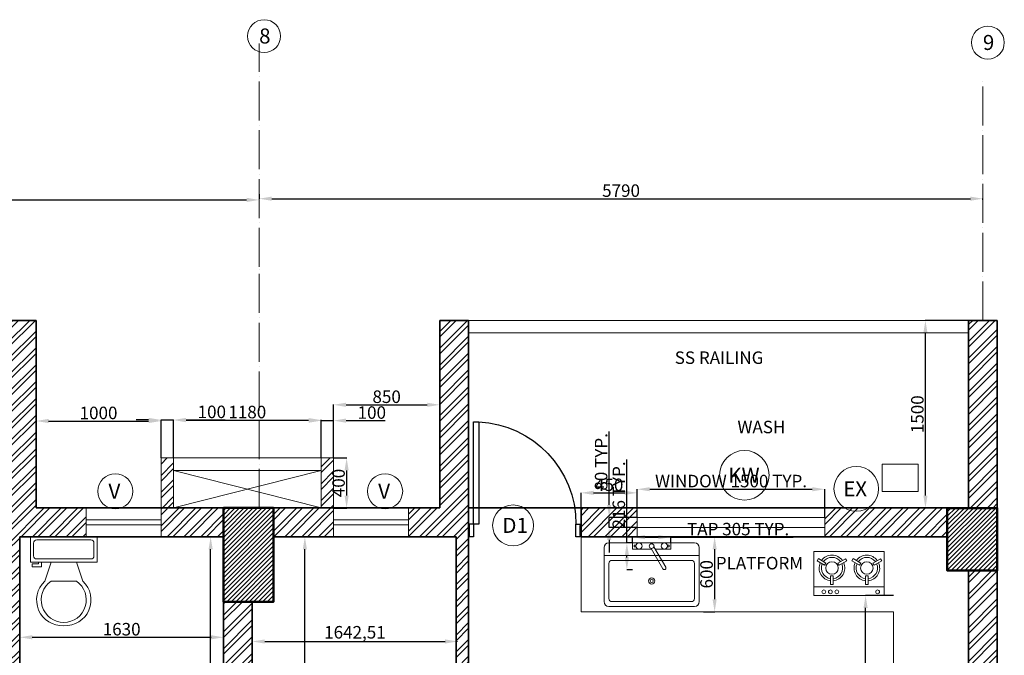
# Model space of a CAD drawing. Units: millimetres. Extents: x -3326 to 29338, y -16792 to 6002.
# Tile 21 of 21: x 21462 to 29338, y 918 to 6002. Entities that reach past the tile are written whole.
import ezdxf

# ---------------------------------------------------------------- set-up
doc = ezdxf.new("R2010")
doc.units = ezdxf.units.MM
doc.header["$PDMODE"] = 35
doc.header["$PDSIZE"] = 5
doc.linetypes.add('ACAD_ISO04W100', pattern=[30, 24, -3, 0, -3])
for name, color, linetype, lineweight in [('A-ANNO-DIMS', 2, 'Continuous', 13), ('A-ANNO-SYMB', 7, 'Continuous', 18), ('A-AREA-IDEN', 7, 'Continuous', 18), ('A-COLS', 1, 'Continuous', 50), ('A-COLS-PATT', 251, 'Continuous', 13), ('A-DOOR', 3, 'Continuous', 25), ('A-EQPM', 9, 'Continuous', 18), ('A-FLOR-CASE', 30, 'Continuous', 18), ('A-FLOR-FIXT', 9, 'Continuous', 18), ('A-FLOR-RAIL', 8, 'Continuous', 20), ('A-FLOR-SHFT', 8, 'Continuous', 18), ('A-GLAZ', 4, 'Continuous', 18), ('A-GRID', 8, 'ACAD_ISO04W100', 13), ('A-GRID-IDEN', 7, 'Continuous', 18), ('A-WALL', 7, 'Continuous', 35), ('A-WALL-PATT', 252, 'Continuous', 13), ('txt', 7, 'Continuous', 18)]:
    doc.layers.add(name, color=color, linetype=linetype, lineweight=lineweight)
doc.styles.get("Standard").update_dxf_attribs({"font": 'arial.ttf'})
doc.dimstyles.new('ISO-25', dxfattribs={"dimtxt": 100, "dimasz": 100, "dimexe": 1.25, "dimexo": 0.625, "dimtad": 1, "dimtxsty": 'Standard', "dimcen": 2.5, "dimadec": 0, "dimazin": 0, "dimtfac": 1, "dimtmove": 0, "dimatfit": 3, "dimfxl": 1, "dimarcsym": 0})
pattern_1 = [(45, (-10476.65, 1e-12), (-67.35192, 67.35192), []), (45, (-10431.74, 1e-12), (-67.35192, 67.35192), [])]

# ---------------------------------------------------------------- blocks, each defined once
blk = doc.blocks.new('A$C0CE462CD')
for p, q in [((860, 100), (860, 0)), ((860, 0), (893.9, 0))]:
    blk.add_line(p, q)
for points in [[(860, 100), (860, 920), (818.4, 920), (818.4, 100)], [(0, 10), (6.1, 10), (6.1, 90), (0, 90)], [(893.9, 10), (900, 10), (900, 90), (893.9, 90)]]:
    blk.add_lwpolyline(points, close=True)
for points in [[(6.1, 0), (40, 0), (40, 100), (6.1, 100)], [(6.1, 100), (6.1, 0)], [(860, 100), (893.9, 100), (893.9, 0)]]:
    blk.add_lwpolyline(points)
blk.add_arc((859.1, 101.9), 819.1, 92.8508, 180.13091)
blk = doc.blocks.new('*U5')
for p, q in [((9.5, -6), (9.5, -2)), ((-10, -8.5), (-8, -8.5)), ((-10, -9.5), (-10, -8.5)), ((-8, -8.5), (-8, -8)), ((-7, -8), (-7, -9.5)), ((-4, -8), (-6, -14)), ((4, -8), (6, -14)), ((-7, -9.5), (-10, -9.5)), ((4, -14), (-4, -14))]:
    blk.add_line(p, q)
blk.add_lwpolyline([(10.5, -8), (10.5, 0), (-10.5, 0), (-10.5, -8)], close=True)
for points in [[(-9.5, -2), (-9.5, -6)], [(8.5, -1), (-8.5, -1)], [(-8.5, -7), (8.5, -7)]]:
    blk.add_lwpolyline(points)
for centre, radius, start, end in [((-8.625, -1.875), 0.8839, 81.8699, 188.1301), ((8.625, -1.875), 0.8839, 351.8699, 98.1301), ((-8.625, -6.125), 0.8839, 171.869898, 278.1301), ((8.625, -6.125), 0.8839, 261.8699, 8.1301), ((-0.4772, -19.9188), 8.0953, 133.01722, 273.38), ((0.0374, -19.8731), 7.127, 124.50543, 269.7), ((-0.0373, -19.8731), 7.127, 270.3, 55.4946), ((0.4773, -19.9188), 8.0953, 266.62, 46.9828)]:
    blk.add_arc(centre, radius, start, end)
blk = doc.blocks.new('Sink-single - 30 in top')
blk.add_line((-15, -3.999996), (15, -3.999996))
for points in [[(-13.5, 0), (13.5, 0)], [(-15, -18.499996), (-15, -1.5)], [(15, -1.5), (15, -18.499996)], [(-12.5, -5.499996), (12.5, -5.499996)], [(-13.5, -17.499996), (-13.5, -6.499996)], [(13.5, -6.499996), (13.5, -17.499996)], [(12.5, -18.499996), (-12.5, -18.499996)], [(13.5, -19.999996), (-13.5, -19.999996)]]:
    blk.add_lwpolyline(points)
for radius in [1, 0.5]:
    blk.add_circle((0, -11.999996), radius)
for centre, radius, start, end in [((-13.5, -1.5), 1.5, 90, 180), ((13.5, -1.5), 1.5, 0, 90), ((-12.5, -6.499996), 1, 90, 180), ((12.5, -6.499996), 1, 0, 90), ((-13.5, -18.499996), 1.5, 180, 270), ((-12.5, -17.499996), 1, 180, 270), ((12.5, -17.499996), 1, 270, 0), ((13.5, -18.499996), 1.5, 270, 0)]:
    blk.add_arc(centre, radius, start, end)
blk = doc.blocks.new('Faucet - kit sink top')
for p, q in [((-5.5, -0.75), (-5.5, -1.25)), ((-4.94278, -0.75), (-5.5, -0.75)), ((-5.5, -1.25), (-4.94278, -1.25)), ((-0.14775, -1.7441), (3.56698, -8.1782)), ((4.43301, -7.6782), (0.71828, -1.2441)), ((4.94278, -0.75), (5.5, -0.75)), ((5.5, -1.25), (4.94278, -1.25)), ((5.5, -0.75), (5.5, -1.25))]:
    blk.add_line(p, q)
blk.add_lwpolyline([(-0.00587, -2), (-6, -2), (-6, 0), (6, 0), (6, -2), (1.15195, -2)])
for centre, radius in [((-4, -1), 1), ((4, -1), 1), ((0, -1), 0.75)]:
    blk.add_circle(centre, radius)
blk.add_arc((4, -7.9282), 0.5, 210, 30)
blk = doc.blocks.new('*D98')
at = {"layer": 'A-ANNO-DIMS', "color": 0, "lineweight": -2, "transparency": 16777216}
for p, q in [((29051.7, 3596), (28706, 3596)), ((28707.2, 2196), (28707.2, 3496)), ((29051.7, 2096), (28706, 2096))]:
    blk.add_line(p, q, dxfattribs=at)
at = {"layer": 'A-ANNO-DIMS', "color": 0, "transparency": 16777216}
for points in [[(28690.6, 3496), (28723.9, 3496), (28707.2, 3596)], [(28690.6, 2196), (28723.9, 2196), (28707.2, 2096)]]:
    blk.add_solid(points, dxfattribs=at)
at = {"layer": 'Defpoints', "color": 0, "transparency": 16777216}
for p in [(28707.2, 3596), (29052.3, 3596), (29052.3, 2096)]:
    blk.add_point(p, dxfattribs=at)
at = {"layer": 'A-ANNO-DIMS', "color": 0, "transparency": 16777216, "insert": (28655.6, 2846), "char_height": 100, "attachment_point": 5, "rotation": 90}
blk.add_mtext('1500', dxfattribs=at)
blk = doc.blocks.new('*D99')
at = {"layer": 'A-ANNO-DIMS', "color": 0, "lineweight": -2, "transparency": 16777216}
for p, q in [((26931, 1866), (27022.1, 1866)), ((27020.9, 1766), (27020.9, 1366)), ((26931, 1266), (27022.1, 1266))]:
    blk.add_line(p, q, dxfattribs=at)
at = {"layer": 'A-ANNO-DIMS', "color": 0, "transparency": 16777216}
for points in [[(27004.2, 1766), (27037.5, 1766), (27020.9, 1866)], [(27004.2, 1366), (27037.5, 1366), (27020.9, 1266)]]:
    blk.add_solid(points, dxfattribs=at)
at = {"layer": 'Defpoints', "color": 0, "transparency": 16777216}
for p in [(26930.3, 1866), (26930.3, 1266), (27020.9, 1266)]:
    blk.add_point(p, dxfattribs=at)
at = {"layer": 'A-ANNO-DIMS', "color": 0, "transparency": 16777216, "insert": (26969.2, 1566), "char_height": 100, "attachment_point": 5, "rotation": 90}
blk.add_mtext('600', dxfattribs=at)
blk = doc.blocks.new('*D103')
at = {"layer": 'A-ANNO-DIMS', "color": 0, "lineweight": -2, "transparency": 16777216}
for p, q in [((28451.7, 1396.4), (28227.4, 1396.4)), ((28228.6, -1834), (28228.6, 1296.4)), ((28451.7, -1934), (28227.4, -1934))]:
    blk.add_line(p, q, dxfattribs=at)
at = {"layer": 'A-ANNO-DIMS', "color": 0, "transparency": 16777216}
for points in [[(28212, 1296.4), (28245.3, 1296.4), (28228.6, 1396.4)], [(28212, -1834), (28245.3, -1834), (28228.6, -1934)]]:
    blk.add_solid(points, dxfattribs=at)
at = {"layer": 'Defpoints', "color": 0, "transparency": 16777216}
for p in [(28228.6, 1396.4), (28452.3, 1396.4), (28452.3, -1934)]:
    blk.add_point(p, dxfattribs=at)
at = {"layer": 'A-ANNO-DIMS', "color": 0, "transparency": 16777216, "insert": (28167.9, -268.8), "char_height": 100, "attachment_point": 5, "rotation": 90}
blk.add_mtext('3330,33', dxfattribs=at)
blk = doc.blocks.new('*D104')
at = {"layer": 'A-ANNO-DIMS', "color": 0, "lineweight": -2, "transparency": 16777216}
for p, q in [((25952.3, 2096.7), (25952.3, 2218.5)), ((26052.3, 2217.2), (26302.3, 2217.2)), ((26402.3, 2096.7), (26402.3, 2218.5))]:
    blk.add_line(p, q, dxfattribs=at)
at = {"layer": 'A-ANNO-DIMS', "color": 0, "transparency": 16777216}
for points in [[(26052.3, 2233.9), (26052.3, 2200.5), (25952.3, 2217.2)], [(26302.3, 2233.9), (26302.3, 2200.5), (26402.3, 2217.2)]]:
    blk.add_solid(points, dxfattribs=at)
at = {"layer": 'Defpoints', "color": 0, "transparency": 16777216}
for p in [(26402.3, 2217.2), (25952.3, 2096), (26402.3, 2096)]:
    blk.add_point(p, dxfattribs=at)
at = {"layer": 'A-ANNO-DIMS', "color": 0, "transparency": 16777216, "insert": (26177.3, 2268.9), "char_height": 100, "attachment_point": 5}
blk.add_mtext('450', dxfattribs=at)
blk = doc.blocks.new('*D105')
at = {"layer": 'A-ANNO-DIMS', "color": 0, "lineweight": -2, "transparency": 16777216}
for p, q in [((22692.3, 2496.7), (22692.3, 2800.2)), ((22792.3, 2799), (23772.3, 2799)), ((23872.3, 2496.7), (23872.3, 2800.2))]:
    blk.add_line(p, q, dxfattribs=at)
at = {"layer": 'A-ANNO-DIMS', "color": 0, "transparency": 16777216}
for points in [[(22792.3, 2815.6), (22792.3, 2782.3), (22692.3, 2799)], [(23772.3, 2815.6), (23772.3, 2782.3), (23872.3, 2799)]]:
    blk.add_solid(points, dxfattribs=at)
at = {"layer": 'Defpoints', "color": 0, "transparency": 16777216}
for p in [(23872.3, 2799), (22692.3, 2496), (23872.3, 2496)]:
    blk.add_point(p, dxfattribs=at)
at = {"layer": 'A-ANNO-DIMS', "color": 0, "transparency": 16777216, "insert": (23282.3, 2850.6), "char_height": 100, "attachment_point": 5}
blk.add_mtext('1180', dxfattribs=at)
blk = doc.blocks.new('*D106')
at = {"layer": 'A-ANNO-DIMS', "color": 0, "lineweight": -2, "transparency": 16777216}
for p, q in [((23772.3, 2794.8), (23672.3, 2794.8)), ((23872.3, 2496.7), (23872.3, 2796)), ((23872.3, 2794.8), (23972.3, 2794.8)), ((23972.3, 2496.7), (23972.3, 2796)), ((24072.3, 2794.8), (24384.7, 2794.8))]:
    blk.add_line(p, q, dxfattribs=at)
at = {"layer": 'A-ANNO-DIMS', "color": 0, "transparency": 16777216}
for points in [[(23772.3, 2811.5), (23772.3, 2778.1), (23872.3, 2794.8)], [(24072.3, 2811.5), (24072.3, 2778.1), (23972.3, 2794.8)]]:
    blk.add_solid(points, dxfattribs=at)
at = {"layer": 'Defpoints', "color": 0, "transparency": 16777216}
for p in [(23972.3, 2794.8), (23872.3, 2496), (23972.3, 2496)]:
    blk.add_point(p, dxfattribs=at)
at = {"layer": 'A-ANNO-DIMS', "color": 0, "transparency": 16777216, "insert": (24278.5, 2846.5), "char_height": 100, "attachment_point": 5}
blk.add_mtext('100', dxfattribs=at)
blk = doc.blocks.new('*D107')
at = {"layer": 'A-ANNO-DIMS', "color": 0, "lineweight": -2, "transparency": 16777216}
for p, q in [((22492.3, 2800.2), (22392.3, 2800.2)), ((22592.3, 2496.7), (22592.3, 2801.5)), ((22592.3, 2800.2), (22692.3, 2800.2)), ((22692.3, 2496.7), (22692.3, 2801.5)), ((22792.3, 2800.2), (23104.7, 2800.2))]:
    blk.add_line(p, q, dxfattribs=at)
at = {"layer": 'A-ANNO-DIMS', "color": 0, "transparency": 16777216}
for points in [[(22492.3, 2816.9), (22492.3, 2783.5), (22592.3, 2800.2)], [(22792.3, 2816.9), (22792.3, 2783.5), (22692.3, 2800.2)]]:
    blk.add_solid(points, dxfattribs=at)
at = {"layer": 'Defpoints', "color": 0, "transparency": 16777216}
for p in [(22692.3, 2800.2), (22592.3, 2496), (22692.3, 2496)]:
    blk.add_point(p, dxfattribs=at)
at = {"layer": 'A-ANNO-DIMS', "color": 0, "transparency": 16777216, "insert": (22998.5, 2851.9), "char_height": 100, "attachment_point": 5}
blk.add_mtext('100', dxfattribs=at)
blk = doc.blocks.new('*D108')
at = {"layer": 'A-ANNO-DIMS', "color": 0, "lineweight": -2, "transparency": 16777216}
for p, q in [((21592.3, 2702.3), (21592.3, 2793.1)), ((21692.3, 2791.9), (22492.3, 2791.9)), ((22592.3, 2702.3), (22592.3, 2793.1))]:
    blk.add_line(p, q, dxfattribs=at)
at = {"layer": 'A-ANNO-DIMS', "color": 0, "transparency": 16777216}
for points in [[(21692.3, 2808.5), (21692.3, 2775.2), (21592.3, 2791.9)], [(22492.3, 2808.5), (22492.3, 2775.2), (22592.3, 2791.9)]]:
    blk.add_solid(points, dxfattribs=at)
at = {"layer": 'Defpoints', "color": 0, "transparency": 16777216}
for p in [(22592.3, 2791.9), (21592.3, 2701.7), (22592.3, 2701.7)]:
    blk.add_point(p, dxfattribs=at)
at = {"layer": 'A-ANNO-DIMS', "color": 0, "transparency": 16777216, "insert": (22092.3, 2843.6), "char_height": 100, "attachment_point": 5}
blk.add_mtext('1000', dxfattribs=at)
blk = doc.blocks.new('*D109')
at = {"layer": 'A-ANNO-DIMS', "color": 0, "lineweight": -2, "transparency": 16777216}
for p, q in [((23972.3, 2647), (23972.3, 2922.7)), ((24072.3, 2921.4), (24722.3, 2921.4)), ((24822.3, 2647), (24822.3, 2922.7))]:
    blk.add_line(p, q, dxfattribs=at)
at = {"layer": 'A-ANNO-DIMS', "color": 0, "transparency": 16777216}
for points in [[(24072.3, 2938.1), (24072.3, 2904.8), (23972.3, 2921.4)], [(24722.3, 2938.1), (24722.3, 2904.8), (24822.3, 2921.4)]]:
    blk.add_solid(points, dxfattribs=at)
at = {"layer": 'Defpoints', "color": 0, "transparency": 16777216}
for p in [(24822.3, 2921.4), (23972.3, 2646.4), (24822.3, 2646.4)]:
    blk.add_point(p, dxfattribs=at)
at = {"layer": 'A-ANNO-DIMS', "color": 0, "transparency": 16777216, "insert": (24397.3, 2973.1), "char_height": 100, "attachment_point": 5}
blk.add_mtext('850', dxfattribs=at)
blk = doc.blocks.new('*D110')
at = {"layer": 'A-ANNO-DIMS', "color": 0, "lineweight": -2, "transparency": 16777216}
for p, q in [((23972.9, 2496), (24078.3, 2496)), ((24077, 2396), (24077, 2196)), ((23972.9, 2096), (24078.3, 2096))]:
    blk.add_line(p, q, dxfattribs=at)
at = {"layer": 'A-ANNO-DIMS', "color": 0, "transparency": 16777216}
for points in [[(24060.4, 2396), (24093.7, 2396), (24077, 2496)], [(24060.4, 2196), (24093.7, 2196), (24077, 2096)]]:
    blk.add_solid(points, dxfattribs=at)
at = {"layer": 'Defpoints', "color": 0, "transparency": 16777216}
for p in [(23972.3, 2496), (23972.3, 2096), (24077, 2096)]:
    blk.add_point(p, dxfattribs=at)
at = {"layer": 'A-ANNO-DIMS', "color": 0, "transparency": 16777216, "insert": (24025.4, 2296), "char_height": 100, "attachment_point": 5, "rotation": 90}
blk.add_mtext('400', dxfattribs=at)
blk = doc.blocks.new('*D111')
at = {"layer": 'A-ANNO-DIMS', "color": 0, "lineweight": -2, "transparency": 16777216}
for p, q in [((23322.3, 1029), (23322.3, 1029.6)), ((23422.3, 1028.4), (24864.8, 1028.4)), ((24964.8, 1029), (24964.8, 1029.6))]:
    blk.add_line(p, q, dxfattribs=at)
at = {"layer": 'A-ANNO-DIMS', "color": 0, "transparency": 16777216}
for points in [[(23422.3, 1045), (23422.3, 1011.7), (23322.3, 1028.4)], [(24864.8, 1045), (24864.8, 1011.7), (24964.8, 1028.4)]]:
    blk.add_solid(points, dxfattribs=at)
at = {"layer": 'Defpoints', "color": 0, "transparency": 16777216}
for p in [(23322.3, 1028.4), (24964.8, 1028.4), (24964.8, 1028.4)]:
    blk.add_point(p, dxfattribs=at)
at = {"layer": 'A-ANNO-DIMS', "color": 0, "transparency": 16777216, "insert": (24143.6, 1089.1), "char_height": 100, "attachment_point": 5}
blk.add_mtext('1642,51', dxfattribs=at)
blk = doc.blocks.new('*D112')
at = {"layer": 'A-ANNO-DIMS', "color": 0, "lineweight": -2, "transparency": 16777216}
for p, q in [((23743.4, 1866), (23744, 1866)), ((23742.8, -1634), (23742.8, 1766)), ((23743.4, -1734), (23744, -1734))]:
    blk.add_line(p, q, dxfattribs=at)
at = {"layer": 'A-ANNO-DIMS', "color": 0, "transparency": 16777216}
for points in [[(23726.1, 1766), (23759.4, 1766), (23742.8, 1866)], [(23726.1, -1634), (23759.4, -1634), (23742.8, -1734)]]:
    blk.add_solid(points, dxfattribs=at)
at = {"layer": 'Defpoints', "color": 0, "transparency": 16777216}
for p in [(23742.8, 1866), (23742.8, 1866), (23742.8, -1734)]:
    blk.add_point(p, dxfattribs=at)
at = {"layer": 'A-ANNO-DIMS', "color": 0, "transparency": 16777216, "insert": (23691.1, 66), "char_height": 100, "attachment_point": 5, "rotation": 90}
blk.add_mtext('3600', dxfattribs=at)
blk = doc.blocks.new('*D113')
at = {"layer": 'A-ANNO-DIMS', "color": 0, "lineweight": -2, "transparency": 16777216}
for p, q in [((21462.3, 1061.3), (21462.3, 1060.7)), ((21562.3, 1061.9), (22992.3, 1061.9)), ((23092.3, 1062.5), (23092.3, 1063.2))]:
    blk.add_line(p, q, dxfattribs=at)
at = {"layer": 'A-ANNO-DIMS', "color": 0, "transparency": 16777216}
for points in [[(21562.3, 1078.6), (21562.3, 1045.3), (21462.3, 1061.9)], [(22992.3, 1078.6), (22992.3, 1045.3), (23092.3, 1061.9)]]:
    blk.add_solid(points, dxfattribs=at)
at = {"layer": 'Defpoints', "color": 0, "transparency": 16777216}
for p in [(21462.3, 1061.9), (23092.3, 1061.9), (23092.3, 1061.9)]:
    blk.add_point(p, dxfattribs=at)
at = {"layer": 'A-ANNO-DIMS', "color": 0, "transparency": 16777216, "insert": (22277.3, 1113.6), "char_height": 100, "attachment_point": 5}
blk.add_mtext('1630', dxfattribs=at)
blk = doc.blocks.new('*D114')
at = {"layer": 'A-ANNO-DIMS', "color": 0, "lineweight": -2, "transparency": 16777216}
for p, q in [((23091.7, 1866), (22987.8, 1866)), ((22989, -834), (22989, 1766)), ((23091.7, -934), (22987.8, -934))]:
    blk.add_line(p, q, dxfattribs=at)
at = {"layer": 'A-ANNO-DIMS', "color": 0, "transparency": 16777216}
for points in [[(22972.4, 1766), (23005.7, 1766), (22989, 1866)], [(22972.4, -834), (23005.7, -834), (22989, -934)]]:
    blk.add_solid(points, dxfattribs=at)
at = {"layer": 'Defpoints', "color": 0, "transparency": 16777216}
for p in [(22989, 1866), (23092.3, 1866), (23092.3, -934)]:
    blk.add_point(p, dxfattribs=at)
at = {"layer": 'A-ANNO-DIMS', "color": 0, "transparency": 16777216, "insert": (22937.4, 466), "char_height": 100, "attachment_point": 5, "rotation": 90}
blk.add_mtext('2800', dxfattribs=at)
blk = doc.blocks.new('*D155')
at = {"layer": 'A-ANNO-DIMS', "color": 0, "lineweight": -2, "transparency": 16777216}
for p, q in [((17397.3, 4561.1), (17397.3, 4561.8)), ((17497.3, 4560.5), (23277.3, 4560.5)), ((23377.3, 4561.1), (23377.3, 4561.8))]:
    blk.add_line(p, q, dxfattribs=at)
at = {"layer": 'A-ANNO-DIMS', "color": 0, "transparency": 16777216}
for points in [[(17497.3, 4577.2), (17497.3, 4543.8), (17397.3, 4560.5)], [(23277.3, 4577.2), (23277.3, 4543.8), (23377.3, 4560.5)]]:
    blk.add_solid(points, dxfattribs=at)
at = {"layer": 'Defpoints', "color": 0, "transparency": 16777216}
for p in [(17397.3, 4560.5), (23377.3, 4560.5), (23377.3, 4560.5)]:
    blk.add_point(p, dxfattribs=at)
at = {"layer": 'A-ANNO-DIMS', "color": 0, "transparency": 16777216, "insert": (20387.3, 4612.2), "char_height": 100, "attachment_point": 5}
blk.add_mtext('5980', dxfattribs=at)
blk = doc.blocks.new('*D156')
at = {"layer": 'A-ANNO-DIMS', "color": 0, "lineweight": -2, "transparency": 16777216}
for p, q in [((23377.3, 4606), (23377.3, 4568.8)), ((23477.3, 4570), (29067.3, 4570)), ((29167.3, 4561.1), (29167.3, 4571.3))]:
    blk.add_line(p, q, dxfattribs=at)
at = {"layer": 'A-ANNO-DIMS', "color": 0, "transparency": 16777216}
for points in [[(23477.3, 4586.7), (23477.3, 4553.4), (23377.3, 4570)], [(29067.3, 4586.7), (29067.3, 4553.4), (29167.3, 4570)]]:
    blk.add_solid(points, dxfattribs=at)
at = {"layer": 'Defpoints', "color": 0, "transparency": 16777216}
for p in [(23377.3, 4606.6), (29167.3, 4570), (29167.3, 4560.5)]:
    blk.add_point(p, dxfattribs=at)
at = {"layer": 'A-ANNO-DIMS', "color": 0, "transparency": 16777216, "insert": (26272.3, 4621.7), "char_height": 100, "attachment_point": 5}
blk.add_mtext('5790', dxfattribs=at)
blk = doc.blocks.new('COOKTOP-TWO-BURNER')
for p, q in [((561.3, 350.8), (0, 350.8)), ((0, 0), (0, 350.8)), ((561.3, 0), (561.3, 350.8)), ((26.1, 276.2), (36.6, 294.4)), ((86.6, 241.2), (26.1, 276.2)), ((97.2, 259.4), (36.6, 294.4)), ((86.6, 241.2), (97.2, 259.4)), ((193, 259.4), (253.6, 294.3)), ((193, 259.4), (203.5, 241.1)), ((203.5, 241.1), (264.1, 276.1)), ((253.6, 294.3), (264.1, 276.1)), ((305, 276.2), (315.6, 294.4)), ((365.6, 241.2), (305, 276.2)), ((376.1, 259.4), (315.6, 294.4)), ((365.6, 241.2), (376.1, 259.4)), ((472, 259.4), (532.5, 294.3)), ((472, 259.4), (482.5, 241.1)), ((482.5, 241.1), (543, 276.1)), ((532.5, 294.3), (543, 276.1)), ((134.5, 158.1), (134.5, 88.2)), ((155.6, 158.1), (134.5, 158.1)), ((155.6, 158.1), (155.5, 88.2)), ((413.5, 158.1), (413.4, 88.2)), ((434.5, 158.1), (413.5, 158.1)), ((434.5, 158.1), (434.5, 88.2)), ((155.5, 88.2), (134.5, 88.2)), ((434.5, 88.2), (413.4, 88.2)), ((561.3, 70.2), (0, 70.2)), ((561.3, 0), (0, 0))]:
    blk.add_line(p, q)
at = {"extrusion": (0, 0, -1)}
for centre, major_axis, start_param, end_param in [((145.1, 219.6), (-0.2, 102.8), -0.942584, 0.946692), ((424, 219.6), (0, 102.8), -0.944011, 0.945266), ((145.1, 219.6), (-0.1, 102.8), 3.2451, 5.134376), ((145.1, 219.6), (-60.3, 60.3), 4.051123, 5.898002), ((145.1, 219.6), (-60.3, 60.3), 6.145519, 7.992397), ((145.1, 219.6), (-35.5, 35.5), 2.356194490192311, 8.639379797371898), ((145.1, 219.6), (0.1, 102.8), 1.148752, 3.038029), ((145.1, 219.6), (60.3, 60.3), 0.385932, 2.23281), ((424, 219.6), (0, 102.8), 3.244173, 5.13345), ((424, 219.6), (60.3, 60.3), 2.480327, 4.327205), ((424, 219.6), (-60.3, 60.3), 6.145519, 7.992397), ((424, 219.6), (-35.5, 35.5), 2.356194490192306, 8.639379797371893), ((424, 219.6), (0.1, 102.8), 1.14879, 3.038067), ((424, 219.6), (60.3, 60.3), 0.385932, 2.23281), ((79.9, 28.7), (-10.8, 10.8), 2.356194490192189, 8.639379797371776), ((132.6, 28.7), (-10.8, 10.8), 2.356194490192189, 8.639379797371776), ((184.2, 28.7), (-10.8, 10.8), 2.356194490192189, 8.639379797371776), ((510, 28.7), (-10.8, 10.8), 2.356194490192189, 8.639379797371776)]:
    blk.add_ellipse(centre, major_axis=major_axis, ratio=1, start_param=start_param, end_param=end_param, dxfattribs=at)
blk = doc.blocks.new('TAG-D1')
blk.add_circle((163.3, 163.3), 163.3)
at = {"insert": (78, 223.5), "char_height": 120, "attachment_point": 1}
blk.add_mtext_dynamic_manual_height_columns('D1', width=137.943, gutter_width=12.5, heights=[0], dxfattribs=at)
blk = doc.blocks.new('TAG-KW')
blk.add_circle((198.2, 198.2), 198.2)
at = {"insert": (70.3, 258.2), "char_height": 120, "attachment_point": 1}
blk.add_mtext_dynamic_manual_height_columns('KW', width=376.575, gutter_width=12.5, heights=[0], dxfattribs=at)
blk = doc.blocks.new('TAG-V')
blk.add_circle((140.7, 140.7), 140.7)
at = {"insert": (85.8, 200.7), "char_height": 120, "attachment_point": 1}
blk.add_mtext_dynamic_manual_height_columns('V', width=129.836, gutter_width=12.5, heights=[0], dxfattribs=at)
blk = doc.blocks.new('GLAZ-600x40')
for p, q in [((600, 40), (0, 40)), ((600, 0), (0, 0))]:
    blk.add_line(p, q)
blk = doc.blocks.new('GLAZ-1500x80')
for p, q in [((0, 80), (1500, 80)), ((0, 0), (1500, 0))]:
    blk.add_line(p, q)
blk = doc.blocks.new('*D207')
at = {"layer": 'A-ANNO-DIMS', "color": 0, "lineweight": -2, "transparency": 16777216}
for p, q in [((26402.3, 2021.7), (26402.3, 2247.3)), ((26502.3, 2246), (27802.3, 2246)), ((27902.3, 2021.7), (27902.3, 2247.3))]:
    blk.add_line(p, q, dxfattribs=at)
at = {"layer": 'A-ANNO-DIMS', "color": 0, "transparency": 16777216}
for points in [[(26502.3, 2262.7), (26502.3, 2229.4), (26402.3, 2246)], [(27802.3, 2262.7), (27802.3, 2229.4), (27902.3, 2246)]]:
    blk.add_solid(points, dxfattribs=at)
at = {"layer": 'Defpoints', "color": 0, "transparency": 16777216}
for p in [(27902.3, 2246), (26402.3, 2021), (27902.3, 2021)]:
    blk.add_point(p, dxfattribs=at)
at = {"layer": 'A-ANNO-DIMS', "color": 0, "transparency": 16777216, "insert": (27152.3, 2298.4), "char_height": 100, "attachment_point": 5}
blk.add_mtext('WINDOW 1500 TYP.', dxfattribs=at)
blk = doc.blocks.new('*D208')
at = {"layer": 'A-ANNO-DIMS', "color": 0, "lineweight": -2, "transparency": 16777216}
for p, q in [((26177.3, 2121), (26177.3, 2709.2)), ((26401.7, 2021), (26176.1, 2021)), ((26177.3, 1941), (26177.3, 2021)), ((26401.7, 1941), (26176.1, 1941)), ((26177.3, 1841), (26177.3, 1741))]:
    blk.add_line(p, q, dxfattribs=at)
at = {"layer": 'A-ANNO-DIMS', "color": 0, "transparency": 16777216}
for points in [[(26160.6, 2121), (26194, 2121), (26177.3, 2021)], [(26160.6, 1841), (26194, 1841), (26177.3, 1941)]]:
    blk.add_solid(points, dxfattribs=at)
at = {"layer": 'Defpoints', "color": 0, "transparency": 16777216}
for p in [(26177.3, 2021), (26402.3, 2021), (26402.3, 1941)]:
    blk.add_point(p, dxfattribs=at)
at = {"layer": 'A-ANNO-DIMS', "color": 0, "transparency": 16777216, "insert": (26125.6, 2465.1), "char_height": 100, "attachment_point": 5, "rotation": 90}
blk.add_mtext('80 TYP.', dxfattribs=at)
blk = doc.blocks.new('*D223')
at = {"layer": 'A-ANNO-DIMS', "color": 0, "lineweight": -2, "transparency": 16777216}
for p, q in [((26364.7, 1817.6), (26364.7, 1863.9)), ((26464.7, 1862.7), (26569.5, 1862.7)), ((26669.5, 1817.6), (26669.5, 1863.9)), ((26669.5, 1862.7), (27648.2, 1862.7))]:
    blk.add_line(p, q, dxfattribs=at)
at = {"layer": 'A-ANNO-DIMS', "color": 0, "transparency": 16777216}
for points in [[(26464.7, 1879.4), (26464.7, 1846), (26364.7, 1862.7)], [(26569.5, 1879.4), (26569.5, 1846), (26669.5, 1862.7)]]:
    blk.add_solid(points, dxfattribs=at)
at = {"layer": 'Defpoints', "color": 0, "transparency": 16777216}
for p in [(26364.7, 1817), (26669.5, 1862.7), (26669.5, 1817)]:
    blk.add_point(p, dxfattribs=at)
at = {"layer": 'A-ANNO-DIMS', "color": 0, "transparency": 16777216, "insert": (27208.8, 1914.4), "char_height": 100, "attachment_point": 5}
blk.add_mtext('TAP 305 TYP.', dxfattribs=at)
blk = doc.blocks.new('*D224')
at = {"layer": 'A-ANNO-DIMS', "color": 0, "lineweight": -2, "transparency": 16777216}
for p, q in [((26318.9, 1817), (26318.9, 2484.4)), ((26364, 1817), (26317.7, 1817)), ((26318.9, 1701.1), (26318.9, 1717)), ((26364, 1601.1), (26317.7, 1601.1))]:
    blk.add_line(p, q, dxfattribs=at)
at = {"layer": 'A-ANNO-DIMS', "color": 0, "transparency": 16777216}
for points in [[(26302.3, 1717), (26335.6, 1717), (26318.9, 1817)], [(26302.3, 1701.1), (26335.6, 1701.1), (26318.9, 1601.1)]]:
    blk.add_solid(points, dxfattribs=at)
at = {"layer": 'Defpoints', "color": 0, "transparency": 16777216}
for p in [(26318.9, 1817), (26364.7, 1817), (26364.7, 1601.1)]:
    blk.add_point(p, dxfattribs=at)
at = {"layer": 'A-ANNO-DIMS', "color": 0, "transparency": 16777216, "insert": (26267.3, 2200.7), "char_height": 100, "attachment_point": 5, "rotation": 90}
blk.add_mtext('216 TYP.', dxfattribs=at)

msp = doc.modelspace()

# ---------------------------------------------------------------- hatches: boundary and pattern name
at = {"layer": 'A-COLS-PATT'}
h = msp.add_hatch(dxfattribs=at)
h.set_pattern_fill('ANSI31', color=256, scale=8)
h.set_pattern_definition([(45, (-18946.33, 12265.585), (-17.960512, 17.960512), [])])
h.paths.add_polyline_path([(23492.301, 2096.048), (23092.301, 2096.048), (23092.301, 1346.048), (23492.301, 1346.048)])
h = msp.add_hatch(dxfattribs=at)
h.set_pattern_fill('ANSI31', color=256, scale=8)
h.set_pattern_definition([(45, (-15733.41, 7308.703), (-17.960512, 17.960512), [])])
h.paths.add_polyline_path([(28882.301, 2095.065), (28882.301, 1595.065), (29282.301, 1595.065), (29282.301, 2095.065)])
at = {"layer": 'A-WALL-PATT'}
h = msp.add_hatch(dxfattribs=at)
h.set_pattern_fill('ANSI32', color=256, scale=10)
h.set_pattern_definition(pattern_1)
h.paths.add_polyline_path([(29282.301, -7283.952), (28882.301, -7283.952), (28882.301, -7383.952), (29052.301, -7383.952), (29052.301, -10763.952), (29282.301, -10763.952)])
h.paths.add_polyline_path([(29282.301, -11263.952), (29052.301, -11263.952), (29052.301, -12763.952), (29282.301, -12763.952)])
h.paths.add_polyline_path([(25052.301, -11263.952), (25652.301, -11263.952), (25652.301, -11123.904), (25652.289, -11123.904), (25652.289, -11033.952), (25052.301, -11033.952), (24572.301, -11033.952), (24572.301, -11263.952), (24822.301, -11263.952), (24822.301, -12763.952), (25052.301, -12763.952)])
h.paths.add_polyline_path([(26902.301, -11033.952), (26552.301, -11033.952), (26552.301, -11263.952), (26902.301, -11263.952)])
h.paths.add_polyline_path([(21992.301, -6683.952), (21362.301, -6683.952), (17512.301, -6683.952), (17512.301, -6783.952), (21362.301, -6783.952), (21992.301, -6783.952)])
h.paths.add_polyline_path([(17512.301, -7283.952), (17282.301, -7283.952), (17282.301, -12163.952), (17512.301, -12163.952), (17512.301, -11263.952), (18112.301, -11263.952), (18112.301, -11033.952), (17512.301, -11033.952)])
h.paths.add_polyline_path([(21462.301, -8211.864), (21462.064, -8211.864), (21462.064, -8142.609), (21462.301, -8133.952), (21362.301, -8133.952), (21362.301, -8233.952), (21362.301, -11033.952), (21162.301, -11033.952), (21162.301, -11263.952), (21362.301, -11263.952), (21362.301, -12763.952), (21592.301, -12763.952), (21592.301, -11263.952), (21992.301, -11263.952), (21992.301, -11033.952), (21592.301, -11033.952), (21462.301, -11033.952)])
h.paths.add_polyline_path([(24152.301, -8133.952), (23322.301, -8133.952), (23322.301, -7433.952), (23092.301, -7433.952), (23092.301, -8133.952), (22241.021, -8133.952), (22241.021, -8142.609), (22241.182, -8142.609), (22241.182, -8211.864), (22241.021, -8233.952), (23092.301, -8233.952), (23092.301, -10513.206), (23322.301, -10513.206), (23322.301, -8233.952), (24152.301, -8233.952)])
h.paths.add_polyline_path([(25052.301, -8233.952), (25052.301, -8133.952), (24952.301, -8133.952), (24952.301, -11033.952), (25052.301, -11033.952)])
h.paths.add_polyline_path([(23972.301, -11033.952), (23493.251, -11033.952), (23493.251, -11263.952), (23972.301, -11263.952)])
h.paths.add_polyline_path([(23092.301, -11033.952), (22592.301, -11033.952), (22592.301, -11263.952), (23092.301, -11263.952)])
h.paths.add_polyline_path([(28882.301, -11033.952), (28702.301, -11033.952), (28702.301, -11263.952), (28882.301, -11263.952)])
h.paths.add_polyline_path([(17512.301, -3883.952), (17387.589, -3883.952), (17387.589, -3888.07), (17282.301, -3888.07), (17282.301, -6683.952), (17512.301, -6683.952)])
h.paths.add_polyline_path([(21462.301, -2183.952), (21362.301, -2183.952), (21362.301, -2383.952), (17282.301, -2383.952), (17282.301, -2483.952), (17512.301, -2483.952), (21462.301, -2483.952)])
h.paths.add_polyline_path([(17512.301, -2483.952), (17282.301, -2483.952), (17282.301, -2833.952), (17512.301, -2833.952)])
h.paths.add_polyline_path([(21462.301, 1866.048), (21992.301, 1866.048), (21992.301, 2096.048), (21592.301, 2096.048), (21592.301, 3596.048), (21362.301, 3596.048), (21362.301, 1866.048), (21362.301, -1283.952), (21462.301, -1283.952)])
h.paths.add_polyline_path([(17512.301, 1496.048), (17282.301, 1496.048), (17282.301, -1983.952), (17612.301, -1983.952), (17612.301, -1883.952), (17512.301, -1883.952)])
h.paths.add_polyline_path([(17512.301, 3596.048), (17282.301, 3596.048), (17282.301, 2096.048), (17512.301, 2096.048)])
h.paths.add_polyline_path([(18135.023, 2096.048), (17685.023, 2096.048), (17685.023, 1866.048), (18135.023, 1866.048), (18135.023, 1876.048), (18128.942, 1876.048), (18128.942, 1956.048), (18135.023, 1956.048)])
h.paths.add_polyline_path([(19385.023, 2096.048), (19035.023, 2096.048), (19035.023, 1866.048), (19385.023, 1866.048)])
h.paths.add_polyline_path([(21362.301, 2096.048), (21185.023, 2096.048), (21185.023, 1866.048), (21362.301, 1866.048)])
h.paths.add_polyline_path([(23092.301, 2096.048), (22592.301, 2096.048), (22592.301, 1866.048), (23092.301, 1866.048)])
h.paths.add_polyline_path([(23972.301, 2096.048), (23492.301, 2096.048), (23492.301, 1866.048), (23972.301, 1866.048)])
h.paths.add_polyline_path([(23972.301, 2496.048), (23872.301, 2496.048), (23872.301, 2096.048), (23972.301, 2096.048)])
h.paths.add_polyline_path([(22692.301, 2496.048), (22592.301, 2496.048), (22592.301, 2096.048), (22692.301, 2096.048)])
h.paths.add_polyline_path([(23322.301, 1346.048), (23092.301, 1346.048), (23092.301, -1733.952), (23322.301, -1733.952)])
h.paths.add_polyline_path([(23092.301, -933.952), (22262.301, -933.952), (22262.301, -1033.952), (23092.301, -1033.952)])
h.paths.add_polyline_path([(24952.301, -1433.952), (24952.301, -1733.952), (23492.301, -1733.952), (23492.301, -1833.952), (24952.301, -1833.952), (24952.301, -2483.952), (25052.301, -2483.952), (25052.301, -2466.23), (25049.26, -2466.23), (25049.26, -2386.23), (25049.941, -1433.952)])
h.paths.add_polyline_path([(22692.301, -11263.952), (22592.301, -11263.952), (22592.301, -11663.952), (22692.301, -11663.952)])
h.paths.add_polyline_path([(23972.301, -11263.952), (23872.301, -11263.952), (23872.301, -11663.952), (23972.301, -11663.952)])
h = msp.add_hatch(dxfattribs=at)
h.set_pattern_fill('ANSI32', color=256, scale=10)
h.set_pattern_definition(pattern_1)
h.paths.add_polyline_path([(29282.301, 3596.048), (29052.301, 3596.048), (29052.301, 2095.065), (29282.301, 2095.065)])
h.paths.add_polyline_path([(25052.301, 3596.048), (24822.301, 3596.048), (24822.301, 2096.048), (24572.301, 2096.048), (24572.301, 1866.048), (24952.301, 1866.048), (24952.301, -633.952), (24972.008, -633.952), (24972.008, -631.026), (25043.379, -631.026), (25052.301, -633.952), (25052.301, 1866.048), (25052.301, 1876.048), (25051.713, 1876.048), (25051.713, 1956.048)])
h.paths.add_polyline_path([(29282.301, 1595.065), (29052.301, 1595.065), (29052.301, -1883.676), (29282.301, -1883.676), (29282.301, 336.048)])
h.paths.add_polyline_path([(28882.301, 2096.048), (27902.301, 2096.048), (27902.301, 1866.048), (28882.301, 1866.048)])
h.paths.add_polyline_path([(26402.301, 2096.048), (25952.301, 2096.048), (25952.301, 1866.048), (26402.301, 1866.048)])
h.paths.add_polyline_path([(28882.301, -2383.952), (25952.301, -2383.952), (25952.301, -2483.952), (27152.301, -2483.952), (27152.301, -2683.952), (27382.301, -2683.952), (27382.301, -2483.952), (28882.301, -2483.952)])

# ---------------------------------------------------------------- linework, layer by layer
at = {"layer": 'A-ANNO-SYMB'}
msp.add_circle((28154.444, 2249.364), 178.636, dxfattribs=at)
at = {"layer": 'A-COLS'}
for points in [[(23092.301, 2096.048), (23492.301, 2096.048), (23492.301, 1346.048), (23092.301, 1346.048)], [(28882.301, 2095.065), (29282.301, 2095.065), (29282.301, 1595.065), (28882.301, 1595.065)]]:
    msp.add_lwpolyline(points, close=True, dxfattribs=at)
at = {"layer": 'A-EQPM'}
msp.add_lwpolyline([(28361.2, 2446.539), (28649.928, 2446.539), (28649.928, 2227.788), (28361.2, 2227.788)], close=True, dxfattribs=at)
at = {"layer": 'A-FLOR-CASE'}
for p, q in [((25952.301, 1866.048), (25952.301, 1266.048)), ((25952.301, 1266.048), (28452.301, 1266.048)), ((28452.301, -1933.952), (28452.301, 1266.048))]:
    msp.add_line(p, q, dxfattribs=at)
at = {"layer": 'A-FLOR-RAIL'}
for p, q in [((29052.301, 3596.048), (25052.301, 3596.048)), ((29052.301, 3496.048), (25052.301, 3496.048))]:
    msp.add_line(p, q, dxfattribs=at)
at = {"layer": 'A-FLOR-SHFT'}
for p, q in [((22592.301, 2096.048), (22592.301, 2496.048)), ((22592.301, 2496.048), (22692.301, 2496.048)), ((22692.301, 2496.048), (22692.301, 2096.048)), ((22692.301, 2496.048), (23872.301, 2496.048)), ((23972.301, 2496.048), (23872.301, 2496.048)), ((23872.301, 2496.048), (23872.301, 2096.048)), ((23972.301, 2096.048), (23972.301, 2496.048)), ((22692.301, 2396.048), (23872.301, 2396.048)), ((22692.301, 2096.048), (23872.301, 2396.048)), ((22692.301, 2396.048), (23872.301, 2096.048))]:
    msp.add_line(p, q, dxfattribs=at)
at = {"layer": 'A-GLAZ'}
for p, q in [((21992.301, 1866.048), (21992.301, 2096.048)), ((22592.301, 1866.048), (22592.301, 2096.048)), ((23972.301, 2096.048), (23972.301, 1866.048)), ((24572.301, 2096.048), (24572.301, 1866.048)), ((26402.301, 2096.048), (26402.301, 1866.048)), ((27902.301, 2096.048), (27902.301, 1866.048))]:
    msp.add_line(p, q, dxfattribs=at)
at = {"layer": 'A-GRID', "ltscale": 13}
for p, q in [((23377.301, 4024.981), (23377.301, 5811.048)), ((29167.301, 3596.048), (29167.301, 5524.981)), ((23377.301, 2096.048), (23377.301, 4024.981))]:
    msp.add_line(p, q, dxfattribs=at)
at = {"layer": 'A-GRID-IDEN'}
for centre, radius in [((23416.837, 5870.271), 131.577), ((29206.755, 5818.449), 131.527)]:
    msp.add_circle(centre, radius, dxfattribs=at)
at = {"layer": 'A-WALL'}
for p, q in [((21592.301, 3596.048), (21362.301, 3596.048)), ((21592.301, 3596.048), (21592.301, 2096.048)), ((24822.301, 3596.048), (24822.301, 2096.048)), ((25052.301, 3596.048), (24822.301, 3596.048)), ((25052.301, 3596.048), (25052.301, 1866.048)), ((29052.301, 3596.048), (29052.301, 2095.065)), ((29052.301, 3596.048), (29282.301, 3596.048)), ((29282.301, 336.048), (29282.301, 3596.048)), ((23092.301, 2096.048), (21592.301, 2096.048)), ((24822.301, 2096.048), (23322.301, 2096.048)), ((29052.301, 2096.048), (25052.301, 2096.048)), ((25952.301, 2096.048), (25952.301, 1866.048)), ((23092.301, 1866.048), (21462.301, 1866.048)), ((21462.301, 1866.048), (21462.301, -1283.952)), ((23092.301, 1866.048), (23092.301, -2483.952)), ((24952.301, 1866.048), (23492.301, 1866.048)), ((24952.301, 1866.048), (24952.301, -633.952)), ((25052.301, 1866.048), (25052.301, -2483.952)), ((28882.301, 1866.048), (25952.301, 1866.048)), ((29052.301, 1595.065), (29052.301, -1883.676)), ((23322.301, 1346.048), (23322.301, -1733.952))]:
    msp.add_line(p, q, dxfattribs=at)

# ---------------------------------------------------------------- block references
at = {"layer": 'A-ANNO-SYMB'}
for name, p in [('TAG-KW', (27060.53, 2159.972)), ('TAG-V', (22086.191, 2088.771)), ('TAG-V', (24243.951, 2088.771)), ('TAG-D1', (25245.189, 1793.582))]:
    msp.add_blockref(name, p, dxfattribs=at)
at = {"layer": 'A-DOOR', "xscale": -1}
msp.add_blockref('A$C0CE462CD', (25951.713, 1866.048), dxfattribs=at)
at = {"layer": 'A-EQPM'}
msp.add_blockref('COOKTOP-TWO-BURNER', (27814.586, 1396.382), dxfattribs=at)
at = {"layer": 'A-FLOR-FIXT', "xscale": 25.4, "yscale": 25.4, "zscale": 25.4}
for name, p in [('*U5', (21814.309, 1866.048)), ('Sink-single - 30 in top', (26517.06, 1816.976)), ('Faucet - kit sink top', (26517.06, 1816.976))]:
    msp.add_blockref(name, p, dxfattribs=at)
at = {"layer": 'A-GLAZ'}
for name, p in [('GLAZ-600x40', (21992.301, 1961.048)), ('GLAZ-600x40', (23972.301, 1961.048)), ('GLAZ-1500x80', (26402.301, 1941.048))]:
    msp.add_blockref(name, p, dxfattribs=at)

# ---------------------------------------------------------------- texts
at = {"layer": 'A-ANNO-SYMB', "insert": (28049.792, 2309.364), "char_height": 120, "attachment_point": 1}
msp.add_mtext_dynamic_manual_height_columns('EX', width=92.17276, gutter_width=12.5, heights=[0], dxfattribs=at)
at = {"layer": 'A-AREA-IDEN', "insert": (27203.631, 2793.605), "char_height": 100, "attachment_point": 1}
msp.add_mtext_dynamic_manual_height_columns('WASH', width=1168.90663, gutter_width=12.5, heights=[0], dxfattribs=at)
at = {"layer": 'A-GRID-IDEN', "char_height": 120, "attachment_point": 1}
for s, heights, insert in [('8', [0], (23377.301, 5931.539)), ('9', [204.477], (29167.301, 5879.718))]:
    msp.add_mtext_dynamic_manual_height_columns(s, width=463.74815, gutter_width=12.5, heights=heights, dxfattribs=dict(at, insert=insert))
at = {"layer": 'txt', "char_height": 100, "attachment_point": 1}
for s, width, insert in [('SS RAILING', 1168.90663, (26701.784, 3348.43)), ('PLATFORM', 441.09946, (27030.206, 1705.147))]:
    msp.add_mtext_dynamic_manual_height_columns(s, width=width, gutter_width=12.5, heights=[0], dxfattribs=dict(at, insert=insert))

# ---------------------------------------------------------------- dimensions: what is measured, and where the dimension line sits
at = {"layer": 'A-ANNO-DIMS'}
for base, p1, p2, picture, middle in [((23377.301, 4560.514), (17397.301, 4560.514), (23377.301, 4560.514), '*D155', (20387.301, 4612.197)), ((29167.301, 4570.02), (23377.301, 4606.584), (29167.301, 4560.514), '*D156', (26272.301, 4621.702)), ((24822.301, 2921.442), (23972.301, 2646.359), (24822.301, 2646.359), '*D109', (24397.301, 2973.124)), ((22692.301, 2800.211), (22592.301, 2496.048), (22692.301, 2496.048), '*D107', (22998.519, 2851.893)), ((23872.301, 2798.961), (22692.301, 2496.048), (23872.301, 2496.048), '*D105', (23282.301, 2850.643)), ((22592.301, 2791.877), (21592.301, 2701.673), (22592.301, 2701.673), '*D108', (22092.301, 2843.56)), ((23972.301, 2794.796), (23872.301, 2496.048), (23972.301, 2496.048), '*D106', (24278.519, 2846.478)), ((26402.301, 2217.201), (25952.301, 2096.048), (26402.301, 2096.048), '*D104', (26177.301, 2268.884)), ((23092.301, 1061.924), (21462.301, 1061.924), (23092.301, 1061.924), '*D113', (22277.301, 1113.64)), ((24964.81, 1028.352), (23322.301, 1028.352), (24964.81, 1028.352), '*D111', (24143.555, 1089.072))]:
    dim = msp.add_linear_dim(base=base, p1=p1, p2=p2, dimstyle='ISO-25', override={"dimclrd": 0, "dimclre": 0, "dimclrt": 0}, dxfattribs=at)
    dim.commit()
    dim.dimension.update_dxf_attribs({"geometry": picture, "text_midpoint": middle})
for base, p1, p2, picture, middle in [((28707.238, 3596.048), (29052.301, 2096.048), (29052.301, 3596.048), '*D98', (28655.555, 2846.048)), ((24077.036, 2096.048), (23972.301, 2496.048), (23972.301, 2096.048), '*D110', (24025.354, 2296.048)), ((22989.037, 1866.048), (23092.301, -933.952), (23092.301, 1866.048), '*D114', (22937.355, 466.048)), ((23742.77, 1866.048), (23742.77, -1733.952), (23742.77, 1866.048), '*D112', (23691.053, 66.048)), ((27020.872, 1266.048), (26930.331, 1866.048), (26930.331, 1266.048), '*D99', (26969.189, 1566.048)), ((28228.622, 1396.382), (28452.301, -1933.952), (28452.301, 1396.382), '*D103', (28167.901, -268.785))]:
    dim = msp.add_linear_dim(base=base, p1=p1, p2=p2, angle=90, dimstyle='ISO-25', override={"dimclrd": 0, "dimclre": 0, "dimclrt": 0}, dxfattribs=at)
    dim.commit()
    dim.dimension.update_dxf_attribs({"geometry": picture, "text_midpoint": middle})
for base, p1, p2, picture, middle in [((26177.301, 2021.048), (26402.301, 1941.048), (26402.301, 2021.048), '*D208', (26125.618, 2465.124)), ((26318.94, 1816.976), (26364.66, 1601.095), (26364.66, 1816.976), '*D224', (26267.257, 2200.685))]:
    dim = msp.add_linear_dim(base=base, p1=p1, p2=p2, angle=90, text='<> TYP.', dimstyle='ISO-25', override={"dimdec": 0, "dimlfac": 1, "dimrnd": 0, "dimzin": 0, "dimdsep": 46, "dimlunit": 2}, dxfattribs=at)
    dim.commit()
    dim.dimension.update_dxf_attribs({"geometry": picture, "text_midpoint": middle})
for base, p1, p2, text, picture, middle in [((27902.301, 2246.048), (26402.301, 2021.048), (27902.301, 2021.048), 'WINDOW <> TYP.', '*D207', (27152.301, 2298.412)), ((26669.46, 1862.696), (26364.66, 1816.976), (26669.46, 1816.976), 'TAP <> TYP.', '*D223', (27208.83, 1914.413))]:
    dim = msp.add_linear_dim(base=base, p1=p1, p2=p2, text=text, dimstyle='ISO-25', override={"dimdec": 0, "dimlfac": 1, "dimrnd": 0, "dimzin": 0, "dimdsep": 46, "dimlunit": 2}, dxfattribs=at)
    dim.commit()
    dim.dimension.update_dxf_attribs({"geometry": picture, "text_midpoint": middle})

doc.saveas('drawing.dxf')
